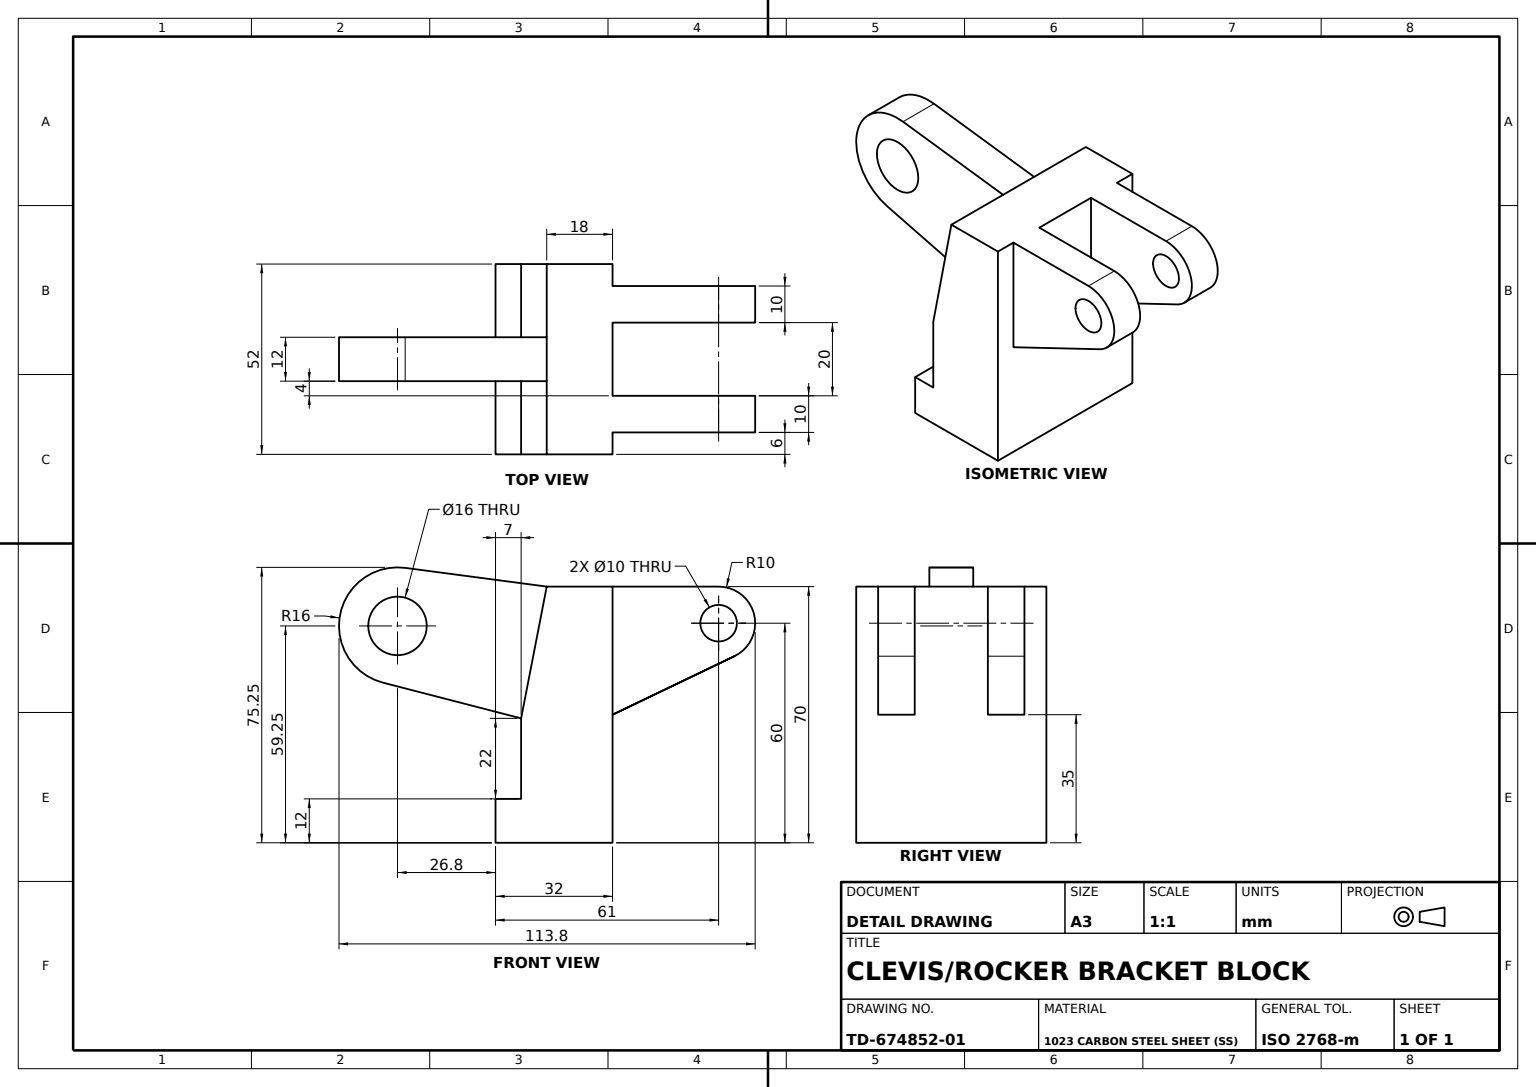
SolidWorks part; units mm, degrees
material "1023 Carbon Steel Sheet (SS)"
ref_plane "Front Plane" through (0, 0, 0) normal (0, 0, 1) x (1, 0, 0)
ref_plane "Top Plane" through (0, 0, 0) normal (0, 1, 0) x (1, 0, 0)
ref_plane "Right Plane" through (0, 0, 0) normal (1, 0, 0) x (0, 0, -1)
sketch "Base Block Sketch" plane through (0, 0, 0) normal (0, 0, 1) x (1, 0, 0)
  line L0 (0, 0) -> (32, 0)
  line L1 (0, 0) -> (0, 12)
  line L2 (0, 12) -> (32, 12)
  line L3 (32, 12) -> (32, 0)
  dimension "D1" = 32
  dimension "D2" = 12
extrude "Base Block" add sketch "Base Block Sketch" along normal blind 52
ref_plane "Plane3" through (0, 0, 0) normal (1, 0, 0) x (0, 0, -1)
ref_plane "Plane4" through (0, 0, 52) normal (0, 0, 1) x (1, 0, 0)
sketch "Upright Profile Sketch" plane through (0, 0, 52) normal (0, 0, 1) x (1, 0, 0)
  line L0 (32, 12) -> (32, 70)
  line L1 (32, 70) -> (14, 70)
  line L3 (32, 12) -> (0, 12) construction
  line L4 (7, 12) -> (7, 34)
  line L6 (7, 34) -> (14, 70)
  line L7 (7, 12) -> (32, 12)
  dimension "D1" = 18
  dimension "D2" = 70
  dimension "D3" = 22
  dimension "D4" = 7
extrude "Upright Body" add sketch "Upright Profile Sketch" against normal blind 52
ref_plane "Plane5" through (0, 0, 6) normal (0, 0, 1) x (1, 0, 0)
sketch "Clevis Lug Sketch" plane through (0, 0, 6) normal (0, 0, 1) x (1, 0, 0)
  line L0 (32, 70) -> (61, 70)
  line L1 (61, 70) -> (61, 60) construction
  line L2 (32, 0) -> (32, 35) construction
  line L3 (32, 70) -> (32, 35)
  line L4 (32, 0) -> (32, 70) construction
  line L5 (32, 35) -> (65.3246, 50.9835)
  arc A0 (65.3246, 50.9835) -> (61, 70) centre (61, 60) ccw
  circle A1 centre (61, 60) radius 5
  dimension "D1" = 20
  dimension "D3" = 10
  dimension "D2" = 61
extrude "Clevis Lug" add sketch "Clevis Lug Sketch" along normal blind 10
ref_plane "Plane6" through (0, 0, 26) normal (0, 0, 1) x (1, 0, 0)
mirror "Clevis Lug Mirror" about plane through (0, 0, 26) normal (0, 0, 1) of "Clevis Lug"
sketch "Pivot Arm Sketch" plane through (0, 0, 26) normal (0, 0, 1) x (1, 0, 0)
  line L0 (7, 12) -> (7, 34) construction
  line L1 (10.5, 52) -> (-26.8014, 59.253)
  line L2 (14, 70) -> (7, 34) construction
  line L3 (14, 70) -> (-24.7051, 75.1151)
  line L4 (7, 34) -> (-30.8017, 43.7612)
  line L5 (14, 70) -> (7, 34)
  arc A0 (-24.7051, 75.1151) -> (-30.8017, 43.7612) centre (-26.8014, 59.253) ccw
  circle A1 centre (-26.8014, 59.253) radius 8
  dimension "D1" = 32
  dimension "D4" = 16
  dimension "D2" = 26.8014
  dimension "D3" = 59.253
extrude "Pivot Arm" add sketch "Pivot Arm Sketch" along normal mid plane 12
